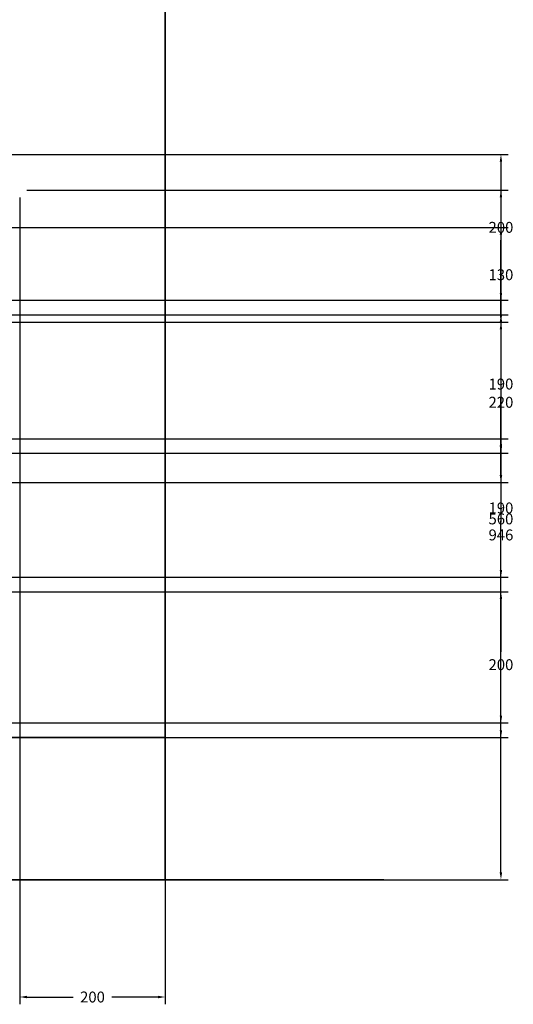
# Model space of a CAD drawing. Units: millimetres. Extents: x 937 to 4561, y 2711 to 5748.
# Tile 6 of 8: x 3829 to 4508, y 2711 to 4062. Entities that reach past the tile are written whole.
import ezdxf

# ---------------------------------------------------------------- set-up
doc = ezdxf.new("R2010")
doc.units = ezdxf.units.MM
doc.header["$MEASUREMENT"] = 0
doc.layers.add('A-ANNO-DIMS', color=2, linetype='Continuous', lineweight=18)
doc.layers.add('A-ELEV', color=7, linetype='Continuous', lineweight=35)
doc.styles.get("Standard").update_dxf_attribs({"font": 'arial.ttf'})
doc.dimstyles.get("Standard").update_dxf_attribs({"dimtxt": 15, "dimasz": 10, "dimexe": 10, "dimexo": 10, "dimgap": 10, "dimtad": 0, "dimtih": 1, "dimtoh": 1, "dimdec": 0, "dimzin": 0, "dimdsep": 46, "dimtxsty": 'Standard', "dimcen": 5, "dimadec": 0, "dimazin": 0, "dimtfac": 1, "dimtdec": 0, "dimtofl": 0, "dimtmove": 0, "dimatfit": 3, "dimfxl": 1, "dimtolj": 1, "dimtzin": 0, "dimarcsym": 0})

# ---------------------------------------------------------------- blocks, each defined once
blk = doc.blocks.new('*D14')
at = {"layer": 'A-ANNO-DIMS', "color": 0, "lineweight": -2, "transparency": 16777216}
for p, q in [((3829.5, 3817.9), (3829.5, 2710.9)), ((4029.5, 3066.9), (4029.5, 2710.9)), ((3839.5, 2720.9), (3902.8, 2720.9)), ((4019.5, 2720.9), (3956.2, 2720.9))]:
    blk.add_line(p, q, dxfattribs=at)
at = {"layer": 'A-ANNO-DIMS', "color": 0, "transparency": 16777216}
for points in [[(3839.5, 2722.6), (3839.5, 2719.2), (3829.5, 2720.9)], [(4019.5, 2722.6), (4019.5, 2719.2), (4029.5, 2720.9)]]:
    blk.add_solid(points, dxfattribs=at)
at = {"layer": 'Defpoints', "color": 0, "transparency": 16777216}
for p in [(3829.5, 3827.9), (4029.5, 3076.9), (4029.5, 2720.9)]:
    blk.add_point(p, dxfattribs=at)
at = {"layer": 'A-ANNO-DIMS', "color": 0, "transparency": 16777216, "insert": (3929.5, 2720.9), "char_height": 15, "attachment_point": 5}
blk.add_mtext('\\A1;200', dxfattribs=at)
blk = doc.blocks.new('*D72')
at = {"layer": 'A-ANNO-DIMS', "color": 0, "lineweight": -2, "transparency": 16777216}
for p, q in [((1764.5, 3646.9), (4500.5, 3646.9)), ((4490.5, 3636.9), (4490.5, 3554.6)), ((4490.5, 3436.9), (4490.5, 3519.2)), ((1764.5, 3426.9), (4500.5, 3426.9))]:
    blk.add_line(p, q, dxfattribs=at)
at = {"layer": 'A-ANNO-DIMS', "color": 0, "transparency": 16777216}
for points in [[(4488.8, 3636.9), (4492.2, 3636.9), (4490.5, 3646.9)], [(4488.8, 3436.9), (4492.2, 3436.9), (4490.5, 3426.9)]]:
    blk.add_solid(points, dxfattribs=at)
at = {"layer": 'Defpoints', "color": 0, "transparency": 16777216}
for p in [(1754.5, 3646.9), (4490.5, 3646.9), (1754.5, 3426.9)]:
    blk.add_point(p, dxfattribs=at)
at = {"layer": 'A-ANNO-DIMS', "color": 0, "transparency": 16777216, "insert": (4490.5, 3536.9), "char_height": 15, "attachment_point": 5}
blk.add_mtext('\\A1;220', dxfattribs=at)
blk = doc.blocks.new('*D73')
at = {"layer": 'A-ANNO-DIMS', "color": 0, "lineweight": -2, "transparency": 16777216}
for p, q in [((1764.5, 3776.9), (4500.5, 3776.9)), ((4490.5, 3766.9), (4490.5, 3729.6)), ((4490.5, 3656.9), (4490.5, 3694.2)), ((1764.5, 3646.9), (4500.5, 3646.9))]:
    blk.add_line(p, q, dxfattribs=at)
at = {"layer": 'A-ANNO-DIMS', "color": 0, "transparency": 16777216}
for points in [[(4488.8, 3766.9), (4492.2, 3766.9), (4490.5, 3776.9)], [(4488.8, 3656.9), (4492.2, 3656.9), (4490.5, 3646.9)]]:
    blk.add_solid(points, dxfattribs=at)
at = {"layer": 'Defpoints', "color": 0, "transparency": 16777216}
for p in [(1754.5, 3776.9), (4490.5, 3776.9), (1754.5, 3646.9)]:
    blk.add_point(p, dxfattribs=at)
at = {"layer": 'A-ANNO-DIMS', "color": 0, "transparency": 16777216, "insert": (4490.5, 3711.9), "char_height": 15, "attachment_point": 5}
blk.add_mtext('\\A1;130', dxfattribs=at)
blk = doc.blocks.new('*D94')
at = {"layer": 'A-ANNO-DIMS', "color": 0, "lineweight": -2, "transparency": 16777216}
for p, q in [((3339.5, 3276.9), (4500.5, 3276.9)), ((4490.5, 3266.9), (4490.5, 3194.6)), ((4490.5, 3086.9), (4490.5, 3159.2)), ((3339.5, 3076.9), (4500.5, 3076.9))]:
    blk.add_line(p, q, dxfattribs=at)
at = {"layer": 'A-ANNO-DIMS', "color": 0, "transparency": 16777216}
for points in [[(4488.8, 3266.9), (4492.2, 3266.9), (4490.5, 3276.9)], [(4488.8, 3086.9), (4492.2, 3086.9), (4490.5, 3076.9)]]:
    blk.add_solid(points, dxfattribs=at)
at = {"layer": 'Defpoints', "color": 0, "transparency": 16777216}
for p in [(3329.5, 3276.9), (4490.5, 3276.9), (3329.5, 3076.9)]:
    blk.add_point(p, dxfattribs=at)
at = {"layer": 'A-ANNO-DIMS', "color": 0, "transparency": 16777216, "insert": (4490.5, 3176.9), "char_height": 15, "attachment_point": 5}
blk.add_mtext('\\A1;200', dxfattribs=at)
blk = doc.blocks.new('*D95')
at = {"layer": 'A-ANNO-DIMS', "color": 0, "lineweight": -2, "transparency": 16777216}
for p, q in [((3319.5, 3486.9), (4500.5, 3486.9)), ((4490.5, 3476.9), (4490.5, 3409.6)), ((4490.5, 3306.9), (4490.5, 3374.2)), ((3319.5, 3296.9), (4500.5, 3296.9))]:
    blk.add_line(p, q, dxfattribs=at)
at = {"layer": 'A-ANNO-DIMS', "color": 0, "transparency": 16777216}
for points in [[(4488.8, 3476.9), (4492.2, 3476.9), (4490.5, 3486.9)], [(4488.8, 3306.9), (4492.2, 3306.9), (4490.5, 3296.9)]]:
    blk.add_solid(points, dxfattribs=at)
at = {"layer": 'Defpoints', "color": 0, "transparency": 16777216}
for p in [(3309.5, 3486.9), (4490.5, 3486.9), (3309.5, 3296.9)]:
    blk.add_point(p, dxfattribs=at)
at = {"layer": 'A-ANNO-DIMS', "color": 0, "transparency": 16777216, "insert": (4490.5, 3391.9), "char_height": 15, "attachment_point": 5}
blk.add_mtext('\\A1;190', dxfattribs=at)
blk = doc.blocks.new('*D96')
at = {"layer": 'A-ANNO-DIMS', "color": 0, "lineweight": -2, "transparency": 16777216}
for p, q in [((3319.5, 3656.9), (4500.5, 3656.9)), ((4490.5, 3646.9), (4490.5, 3579.6)), ((4490.5, 3476.9), (4490.5, 3544.2)), ((3319.5, 3466.9), (4500.5, 3466.9))]:
    blk.add_line(p, q, dxfattribs=at)
at = {"layer": 'A-ANNO-DIMS', "color": 0, "transparency": 16777216}
for points in [[(4488.8, 3646.9), (4492.2, 3646.9), (4490.5, 3656.9)], [(4488.8, 3476.9), (4492.2, 3476.9), (4490.5, 3466.9)]]:
    blk.add_solid(points, dxfattribs=at)
at = {"layer": 'Defpoints', "color": 0, "transparency": 16777216}
for p in [(3309.5, 3656.9), (4490.5, 3656.9), (3309.5, 3466.9)]:
    blk.add_point(p, dxfattribs=at)
at = {"layer": 'A-ANNO-DIMS', "color": 0, "transparency": 16777216, "insert": (4490.5, 3561.9), "char_height": 15, "attachment_point": 5}
blk.add_mtext('\\A1;190', dxfattribs=at)
blk = doc.blocks.new('*D97')
at = {"layer": 'A-ANNO-DIMS', "color": 0, "lineweight": -2, "transparency": 16777216}
for p, q in [((3339.5, 3876.9), (4500.5, 3876.9)), ((4490.5, 3866.9), (4490.5, 3794.6)), ((4490.5, 3686.9), (4490.5, 3759.2)), ((3339.5, 3676.9), (4500.5, 3676.9))]:
    blk.add_line(p, q, dxfattribs=at)
at = {"layer": 'A-ANNO-DIMS', "color": 0, "transparency": 16777216}
for points in [[(4488.8, 3866.9), (4492.2, 3866.9), (4490.5, 3876.9)], [(4488.8, 3686.9), (4492.2, 3686.9), (4490.5, 3676.9)]]:
    blk.add_solid(points, dxfattribs=at)
at = {"layer": 'Defpoints', "color": 0, "transparency": 16777216}
for p in [(3329.5, 3876.9), (4490.5, 3876.9), (3329.5, 3676.9)]:
    blk.add_point(p, dxfattribs=at)
at = {"layer": 'A-ANNO-DIMS', "color": 0, "transparency": 16777216, "insert": (4490.5, 3776.9), "char_height": 15, "attachment_point": 5}
blk.add_mtext('\\A1;200', dxfattribs=at)
blk = doc.blocks.new('*D98')
at = {"layer": 'A-ANNO-DIMS', "color": 0, "lineweight": -2, "transparency": 16777216}
for p, q in [((3019.5, 3656.9), (4500.5, 3656.9)), ((4490.5, 3646.9), (4490.5, 3394.6)), ((4490.5, 3106.9), (4490.5, 3359.2)), ((3019.5, 3096.9), (4500.5, 3096.9))]:
    blk.add_line(p, q, dxfattribs=at)
at = {"layer": 'A-ANNO-DIMS', "color": 0, "transparency": 16777216}
for points in [[(4488.8, 3646.9), (4492.2, 3646.9), (4490.5, 3656.9)], [(4488.8, 3106.9), (4492.2, 3106.9), (4490.5, 3096.9)]]:
    blk.add_solid(points, dxfattribs=at)
at = {"layer": 'Defpoints', "color": 0, "transparency": 16777216}
for p in [(3009.5, 3656.9), (4490.5, 3656.9), (3009.5, 3096.9)]:
    blk.add_point(p, dxfattribs=at)
at = {"layer": 'A-ANNO-DIMS', "color": 0, "transparency": 16777216, "insert": (4490.5, 3376.9), "char_height": 15, "attachment_point": 5}
blk.add_mtext('\\A1;560', dxfattribs=at)
blk = doc.blocks.new('*D102')
at = {"layer": 'A-ANNO-DIMS', "color": 0, "lineweight": -2, "transparency": 16777216}
for p, q in [((3839.5, 3827.9), (4500.5, 3827.9)), ((4490.5, 3817.9), (4490.5, 3372.6)), ((4490.5, 2891.9), (4490.5, 3337.2)), ((4039.5, 2881.9), (4500.5, 2881.9))]:
    blk.add_line(p, q, dxfattribs=at)
at = {"layer": 'A-ANNO-DIMS', "color": 0, "transparency": 16777216}
for points in [[(4488.8, 3817.9), (4492.2, 3817.9), (4490.5, 3827.9)], [(4488.8, 2891.9), (4492.2, 2891.9), (4490.5, 2881.9)]]:
    blk.add_solid(points, dxfattribs=at)
at = {"layer": 'Defpoints', "color": 0, "transparency": 16777216}
for p in [(3829.5, 3827.9), (4490.5, 3827.9), (4029.5, 2881.9)]:
    blk.add_point(p, dxfattribs=at)
at = {"layer": 'A-ANNO-DIMS', "color": 0, "transparency": 16777216, "insert": (4490.5, 3354.9), "char_height": 15, "attachment_point": 5}
blk.add_mtext('\\A1;946', dxfattribs=at)

msp = doc.modelspace()

# ---------------------------------------------------------------- linework, layer by layer
at = {"layer": 'A-ELEV'}
for p, q in [((4029.4852, 3076.9013), (4029.4852, 5476.9013)), ((4029.4852, 2881.9013), (4029.4852, 3876.9013)), ((1429.4852, 3076.9013), (4029.4852, 3076.9013)), ((1429.4852, 2881.9013), (4029.4852, 2881.9013)), ((4029.4852, 2881.9013), (4329.4852, 2881.9013))]:
    msp.add_line(p, q, dxfattribs=at)

# ---------------------------------------------------------------- dimensions: what is measured, and where the dimension line sits
at = {"layer": 'A-ANNO-DIMS'}
for base, p1, p2, picture, middle in [((4490.4852, 3876.9013), (3329.4852, 3676.9013), (3329.4852, 3876.9013), '*D97', (4490.4852, 3776.9013)), ((4490.4852, 3827.9001), (4029.4852, 2881.9013), (3829.4852, 3827.9001), '*D102', (4490.4852, 3354.9007)), ((4490.4852, 3776.9013), (1754.4852, 3646.9013), (1754.4852, 3776.9013), '*D73', (4490.4852, 3711.9013)), ((4490.4852, 3656.9013), (3009.4852, 3096.9013), (3009.4852, 3656.9013), '*D98', (4490.4852, 3376.9013)), ((4490.4852, 3656.9013), (3309.4852, 3466.9013), (3309.4852, 3656.9013), '*D96', (4490.4852, 3561.9013)), ((4490.4852, 3646.9013), (1754.4852, 3426.9013), (1754.4852, 3646.9013), '*D72', (4490.4852, 3536.9013)), ((4490.4852, 3486.9013), (3309.4852, 3296.9013), (3309.4852, 3486.9013), '*D95', (4490.4852, 3391.9013)), ((4490.4852, 3276.9013), (3329.4852, 3076.9013), (3329.4852, 3276.9013), '*D94', (4490.4852, 3176.9013))]:
    dim = msp.add_linear_dim(base=base, p1=p1, p2=p2, angle=90, dimstyle='Standard', override={"dimdec": 0, "dimlfac": 1, "dimrnd": 0, "dimzin": 0, "dimdsep": 46, "dimlunit": 2}, dxfattribs=at)
    dim.commit()
    dim.dimension.update_dxf_attribs({"geometry": picture, "text_midpoint": middle})
dim = msp.add_linear_dim(base=(4029.4852, 2720.9013), p1=(3829.4852, 3827.9001), p2=(4029.4852, 3076.9013), dimstyle='Standard', override={"dimdec": 0, "dimlfac": 1, "dimrnd": 0, "dimzin": 0, "dimdsep": 46, "dimlunit": 2}, dxfattribs=at)
dim.commit()
dim.dimension.update_dxf_attribs({"geometry": '*D14', "text_midpoint": (3929.4852, 2720.9013)})

doc.saveas('drawing.dxf')
